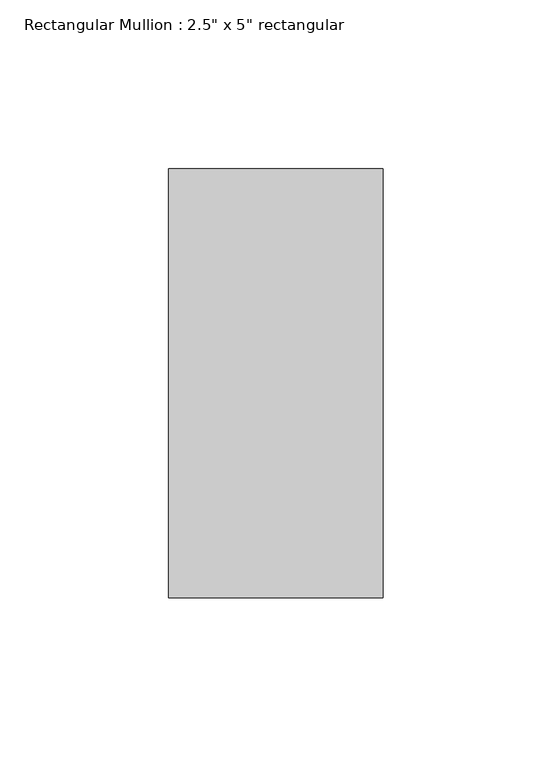
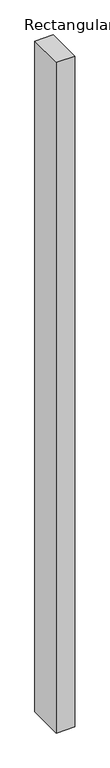
"""IFC4 building model written with IfcOpenShell, lengths in millimetres: member geometry."""

from ifc_helpers import new_model, si_unit, frame, origin, place, context, project, spatial, polyline, outline, extrude, source, transform, mapped, element, save


def member_b030ebd8(model_context):
    return source(origin(), model_context, "Body", "SweptSolid", [
        extrude(outline(polyline([(0.0, 63.5), (0.0, -63.5), (-63.5, -63.5), (-63.5, 63.5), (0.0, 63.5)])), frame((0.0, 0.0, -2432.05), z_axis=(0.0, 0.0, 1.0), x_axis=(1.0, 0.0, 0.0)), (0.0, 0.0, 1.0), 2432.05),
    ])


if __name__ == "__main__":
    model = new_model("IFC4")
    model_context = context("Model", 3, world=origin())
    ifc_project = project(units=[si_unit("LENGTHUNIT", "METRE", prefix="MILLI")], contexts=[model_context])
    site = spatial("IfcSite", under=ifc_project)
    building = spatial("IfcBuilding", under=site)
    placement = place(None, origin())
    member_shape = member_b030ebd8(model_context)
    element("IfcMember", 1, ObjectType="Rectangular Mullion : 2.5\" x 5\" rectangular", at=placement, inside=building, context=model_context, shape_type="MappedRepresentation", body=[
        mapped(member_shape, transform((0.0, 0.0, 0.0), x_axis=(1.0, 0.0, 0.0), y_axis=(0.0, 1.0, 0.0), z_axis=(0.0, 0.0, 1.0))),
    ])
    save(model, "model.ifc")

# Revit data of these elements
# Type "Rectangular Mullion : 2.5\" x 5\" rectangular"
#   built-in parameter 1007304 = 0.416667 (stored number, unit not read)
#   built-in parameter 1007301 = 0.104167 (stored number, unit not read)
#   built-in parameter 1007300 = 0.104167 (stored number, unit not read)
# Element 1 (IfcMember, "Rectangular Mullion : 2.5\" x 5\" rectangular")
#   Materials on its faces: "Aluminum"
# Materials
#   "Aluminum": class "Metal", colour RGB 247 247 247, transparency 0, Description = "Aluminum 6061", Cost = 0
